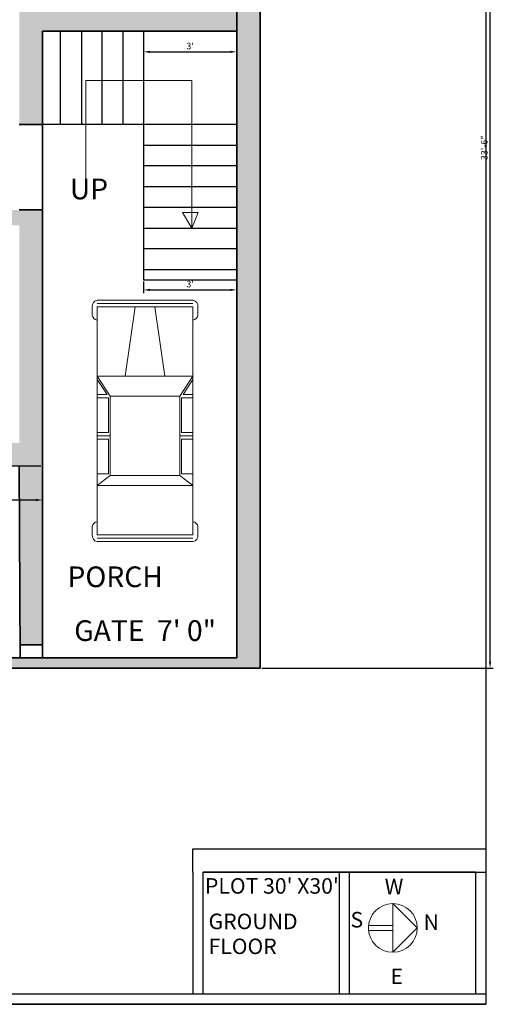
# Model space of a CAD drawing. Units: inches. Extents: x 2341 to 2872, y 1788 to 2419.
# Tile 2 of 3: x 2689 to 2872, y 1813 to 2194. Entities that reach past the tile are written whole.
import ezdxf

# ---------------------------------------------------------------- set-up
doc = ezdxf.new("R2010")
doc.units = ezdxf.units.IN
for name, color, linetype, lineweight in [('A-ANNO-DIMS', 2, 'Continuous', 18), ('A-ANNO-SYMB', 7, 'Continuous', 18), ('A-ANNO-TEXT', 7, 'Continuous', 25), ('A-ANNO-TTLB', 7, 'Continuous', 25), ('A-AREA-IDEN', 7, 'Continuous', 25), ('A-EQPM-VEHI', 8, 'Continuous', 13), ('A-FLOR-STRS', 7, 'Continuous', 25), ('A-WALL', 7, 'Continuous', 35)]:
    doc.layers.add(name, color=color, linetype=linetype, lineweight=lineweight)
doc.layers.add('A-WALL-PATT', color=18, linetype='Continuous', lineweight=13, true_color=0x000000)
doc.styles.get("Standard").update_dxf_attribs({"font": 'arial.ttf'})
doc.dimstyles.new('Copy of ISO-25', dxfattribs={"dimtxt": 2.5, "dimasz": 2.5, "dimexe": 1.25, "dimexo": 0.625, "dimtad": 1, "dimdec": 1, "dimlunit": 4, "dimtxsty": 'Standard', "dimcen": 2.5, "dimadec": 0, "dimazin": 0, "dimtfac": 1, "dimtdec": 1, "dimtmove": 0, "dimatfit": 3, "dimfxl": 1, "dimarcsym": 0})

# ---------------------------------------------------------------- blocks, each defined once
blk = doc.blocks.new('*U6')
for p, q in [((138, 1075), (308, 1075)), ((4818, 1075), (4649, 1075)), ((3, -10), (3, 974)), ((70, -10), (70, 973)), ((138, 973), (410, 973)), ((138, -10), (138, 971)), ((410, 973), (4581, 973)), ((1563, -10), (1563, 973)), ((1563, 973), (1969, 702)), ((1630, 973), (1936, 769)), ((1936, 769), (1936, 973)), ((2003, 973), (2003, 736)), ((2716, 736), (2716, 973)), ((2783, 702), (2783, 973)), ((2851, 973), (2851, 736)), ((3563, 736), (3563, 973)), ((3597, 702), (3801, 973)), ((3801, -10), (3801, 973)), ((4818, 973), (4547, 973)), ((4818, -10), (4818, 971)), ((4886, -10), (4886, 973)), ((4954, -10), (4954, 974)), ((1969, 702), (3597, 702)), ((1969, -10), (1969, 702)), ((2003, 736), (2716, 736)), ((2851, 736), (3563, 736)), ((3597, -10), (3597, 702)), ((138, 193), (1563, 396)), ((3, -11), (3, -995)), ((70, -10), (70, -994)), ((138, -11), (138, -992)), ((1563, -10), (1563, -994)), ((1969, -10), (1969, -723)), ((3597, -10), (3597, -723)), ((3801, -10), (3801, -994)), ((4818, -11), (4818, -992)), ((4886, -10), (4886, -994)), ((4954, -11), (4954, -995)), ((138, -214), (1563, -417)), ((1563, -994), (1969, -723)), ((1630, -994), (1936, -790)), ((1936, -790), (1936, -994)), ((1969, -723), (3597, -723)), ((2003, -994), (2003, -757)), ((2003, -757), (2716, -757)), ((2716, -757), (2716, -994)), ((2783, -723), (2783, -994)), ((2851, -757), (3563, -757)), ((2851, -994), (2851, -757)), ((3563, -757), (3563, -994)), ((3597, -723), (3801, -994)), ((138, -994), (410, -994)), ((410, -994), (4581, -994)), ((4818, -994), (4547, -994)), ((138, -1096), (308, -1096)), ((4818, -1096), (4649, -1096))]:
    blk.add_line(p, q)
for centre, radius, start, end in [((128, 946), 129, 85.6455, 168.0943), ((291, 956), 120, 8.1301, 81.87), ((4665, 956), 120, 98.13, 171.8699), ((4828, 946), 129, 11.9057, 94.3545), ((128, -967), 129, 191.9057, 274.3545), ((291, -977), 120, 278.13, 351.8699), ((4665, -977), 120, 188.1301, 261.87), ((4828, -967), 129, 265.6455, 348.0943)]:
    blk.add_arc(centre, radius, start, end)
blk = doc.blocks.new('*D21')
at = {"layer": 'A-ANNO-DIMS', "color": 0, "lineweight": -2, "transparency": 16777216}
for p, q in [((2556.55, 2020.39), (2556.55, 2006.73)), ((2697.55, 2020.39), (2697.55, 2006.73)), ((2559.05, 2007.98), (2695.05, 2007.98))]:
    blk.add_line(p, q, dxfattribs=at)
at = {"layer": 'A-ANNO-DIMS', "color": 0, "transparency": 16777216}
for points in [[(2559.05, 2008.4), (2559.05, 2007.57), (2556.55, 2007.98)], [(2695.05, 2008.4), (2695.05, 2007.57), (2697.55, 2007.98)]]:
    blk.add_solid(points, dxfattribs=at)
at = {"layer": 'Defpoints', "color": 0, "transparency": 16777216}
for p in [(2556.55, 2021.02), (2697.55, 2021.02), (2697.55, 2007.98)]:
    blk.add_point(p, dxfattribs=at)
at = {"layer": 'A-ANNO-DIMS', "color": 0, "transparency": 16777216, "insert": (2627.05, 2009.89), "char_height": 2.5, "attachment_point": 5}
blk.add_mtext('11\'-9"', dxfattribs=at)
blk = doc.blocks.new('*D22')
at = {"layer": 'A-ANNO-DIMS', "color": 0, "lineweight": -2, "transparency": 16777216}
for p, q in [((2696.93, 2021.02), (2680.85, 2021.02)), ((2682.1, 1949.52), (2682.1, 2018.52)), ((2696.93, 1947.02), (2680.85, 1947.02))]:
    blk.add_line(p, q, dxfattribs=at)
at = {"layer": 'A-ANNO-DIMS', "color": 0, "transparency": 16777216}
for points in [[(2681.68, 2018.52), (2682.52, 2018.52), (2682.1, 2021.02)], [(2681.68, 1949.52), (2682.52, 1949.52), (2682.1, 1947.02)]]:
    blk.add_solid(points, dxfattribs=at)
at = {"layer": 'Defpoints', "color": 0, "transparency": 16777216}
for p in [(2682.1, 2021.02), (2697.55, 2021.02), (2697.55, 1947.02)]:
    blk.add_point(p, dxfattribs=at)
at = {"layer": 'A-ANNO-DIMS', "color": 0, "transparency": 16777216, "insert": (2680.2, 1984.02), "char_height": 2.5, "attachment_point": 5, "rotation": 90}
blk.add_mtext('6\'-2"', dxfattribs=at)
blk = doc.blocks.new('*D27')
at = {"layer": 'A-ANNO-DIMS', "color": 0, "lineweight": -2, "transparency": 16777216}
for p, q in [((2736.55, 2092.39), (2736.55, 2087.89)), ((2772.55, 2092.39), (2772.55, 2087.89)), ((2739.05, 2089.14), (2770.05, 2089.14))]:
    blk.add_line(p, q, dxfattribs=at)
at = {"layer": 'A-ANNO-DIMS', "color": 0, "transparency": 16777216}
for points in [[(2739.05, 2089.56), (2739.05, 2088.72), (2736.55, 2089.14)], [(2770.05, 2089.56), (2770.05, 2088.72), (2772.55, 2089.14)]]:
    blk.add_solid(points, dxfattribs=at)
at = {"layer": 'Defpoints', "color": 0, "transparency": 16777216}
for p in [(2736.55, 2093.02), (2772.55, 2093.02), (2772.55, 2089.14)]:
    blk.add_point(p, dxfattribs=at)
at = {"layer": 'A-ANNO-DIMS', "color": 0, "transparency": 16777216, "insert": (2754.55, 2091.04), "char_height": 2.5, "attachment_point": 5}
blk.add_mtext("3'", dxfattribs=at)
blk = doc.blocks.new('*D28')
at = {"layer": 'A-ANNO-DIMS', "color": 0, "lineweight": -2, "transparency": 16777216}
for p, q in [((2736.55, 2188.39), (2736.55, 2179.85)), ((2772.55, 2188.39), (2772.55, 2179.85)), ((2739.05, 2181.1), (2770.05, 2181.1))]:
    blk.add_line(p, q, dxfattribs=at)
at = {"layer": 'A-ANNO-DIMS', "color": 0, "transparency": 16777216}
for points in [[(2739.05, 2181.51), (2739.05, 2180.68), (2736.55, 2181.1)], [(2770.05, 2181.51), (2770.05, 2180.68), (2772.55, 2181.1)]]:
    blk.add_solid(points, dxfattribs=at)
at = {"layer": 'Defpoints', "color": 0, "transparency": 16777216}
for p in [(2736.55, 2189.02), (2772.55, 2189.02), (2772.55, 2181.1)]:
    blk.add_point(p, dxfattribs=at)
at = {"layer": 'A-ANNO-DIMS', "color": 0, "transparency": 16777216, "insert": (2754.55, 2183), "char_height": 2.5, "attachment_point": 5}
blk.add_mtext("3'", dxfattribs=at)
blk = doc.blocks.new('*D35')
at = {"layer": 'A-ANNO-DIMS', "color": 0, "lineweight": -2, "transparency": 16777216}
for p, q in [((2782.18, 2345.02), (2871.62, 2345.02)), ((2870.37, 1945.52), (2870.37, 2342.52)), ((2782.18, 1943.02), (2871.62, 1943.02))]:
    blk.add_line(p, q, dxfattribs=at)
at = {"layer": 'A-ANNO-DIMS', "color": 0, "transparency": 16777216}
for points in [[(2869.95, 2342.52), (2870.78, 2342.52), (2870.37, 2345.02)], [(2869.95, 1945.52), (2870.78, 1945.52), (2870.37, 1943.02)]]:
    blk.add_solid(points, dxfattribs=at)
at = {"layer": 'Defpoints', "color": 0, "transparency": 16777216}
for p in [(2781.55, 2345.02), (2870.37, 2345.02), (2781.55, 1943.02)]:
    blk.add_point(p, dxfattribs=at)
at = {"layer": 'A-ANNO-DIMS', "color": 0, "transparency": 16777216, "insert": (2868.46, 2144.02), "char_height": 2.5, "attachment_point": 5, "rotation": 90}
blk.add_mtext('33\'-6"', dxfattribs=at)

msp = doc.modelspace()

# ---------------------------------------------------------------- hatches: boundary and pattern name
at = {"layer": 'A-WALL-PATT'}
h = msp.add_hatch(color=256, dxfattribs=at)
h.dxf.hatch_style = 1
h.paths.add_polyline_path([(2781.55, 2345.02), (2421.55, 2345.02), (2421.55, 1985.02), (2421.55, 1949.02), (2421.55, 1943.02), (2781.55, 1943.02), (2781.55, 1985.02)])
h.paths.add_polyline_path([(2550.55, 2336.02), (2772.55, 2336.02), (2772.55, 1994.02), (2772.55, 1985.02), (2772.55, 1947.02), (2430.55, 1947.02), (2430.55, 1985.02), (2454.55, 1985.02), (2454.55, 1994.02), (2430.55, 1994.02), (2430.55, 2114.02), (2496.55, 2114.02), (2514.55, 2114.02), (2514.55, 2120.02), (2496.55, 2120.02), (2496.55, 2168.02), (2556.55, 2168.02), (2556.55, 2174.02), (2550.55, 2174.02), (2478.55, 2174.02), (2478.55, 2170.02), (2490.55, 2170.02), (2490.55, 2168.02), (2490.55, 2120.02), (2430.55, 2120.02), (2430.55, 2168.02), (2430.55, 2174.02), (2430.55, 2204.02), (2430.55, 2336.02)], flags=16)
h.paths.add_polyline_path([(2556.55, 2336.02), (2652.55, 2336.02), (2652.55, 2198.02), (2646.55, 2198.02), (2601.55, 2198.02), (2595.55, 2198.02), (2595.55, 2240.02), (2556.55, 2240.02), (2556.55, 2246.02), (2556.55, 2294.02)], flags=0)
h.paths.add_polyline_path([(2556.55, 2300.02), (2646.55, 2300.02), (2646.55, 2294.02), (2646.55, 2204.02), (2601.55, 2204.02), (2601.55, 2246.02), (2601.55, 2294.02), (2613.55, 2294.02), (2613.55, 2300.02), (2592.55, 2300.02), (2592.55, 2294.02), (2595.55, 2294.02), (2595.55, 2246.02), (2556.55, 2246.02), (2556.55, 2282.02)], flags=0)
h.paths.add_polyline_path([(2680.26, 2307.06), (2747.77, 2307.06), (2747.77, 2329.57), (2770.28, 2329.57), (2770.28, 2307.06), (2770.28, 2239.54), (2770.28, 2217.04), (2747.77, 2217.04), (2747.77, 2239.54), (2680.26, 2239.54)], flags=0)
h.paths.add_polyline_path([(2681.16, 2306.16), (2769.38, 2306.16), (2769.38, 2240.44), (2704.56, 2240.44, -0.009128), (2703.54, 2240.44), (2681.16, 2240.44)], flags=0)
h.paths.add_polyline_path([(2744.14, 2298.19), (2744.14, 2293.47), (2696.44, 2293.47), (2696.44, 2242.73, -0.092104), (2691.71, 2247), (2691.71, 2298.19)], flags=0)
h.paths.add_polyline_path([(2694.86, 2296.62), (2694.86, 2295.04), (2693.29, 2295.04), (2693.29, 2296.62)], flags=0)
h.paths.add_polyline_path([(2478.55, 2173.02), (2478.55, 2172.02), (2478.55, 2171.02), (2442.55, 2171.02), (2442.55, 2170.02), (2438.98, 2170.02), (2430.55, 2170.02), (2430.55, 2174.02), (2442.55, 2174.02), (2442.55, 2173.02)], flags=0)
h.paths.add_polyline_path([(2688.55, 2198.02), (2697.55, 2198.02), (2772.55, 2198.02), (2772.55, 2189.02), (2772.55, 2153.02), (2755.26, 2153.02), (2755.26, 2145.02), (2772.55, 2145.02), (2772.55, 2137.02), (2755.26, 2137.02), (2755.26, 2129.02), (2772.55, 2129.02), (2772.55, 2121.02), (2755.26, 2121.02), (2755.26, 2119.07), (2757.66, 2119.07), (2755.26, 2113.02), (2772.55, 2113.02), (2772.55, 2105.02), (2736.55, 2105.02), (2736.55, 2153.02), (2697.55, 2153.02), (2697.55, 2021.02), (2697.55, 1952.02), (2688.89, 1952.02), (2688.89, 1947.02), (2688.59, 2021.02), (2688.55, 2021.02), (2580.55, 2021.02), (2580.55, 2030.02), (2556.55, 2030.02), (2556.55, 2114.02), (2580.55, 2114.02), (2580.55, 2120.02), (2664.55, 2120.02), (2688.55, 2120.02), (2688.55, 2189.02)], flags=0)
h.paths.add_polyline_path([(2510.86, 2109.17, -0.414214), (2512.75, 2107.25), (2512.59, 2085.13, -0.414214), (2511.43, 2083.99), (2508, 2084.02, -0.414214), (2506.86, 2085.17), (2487.78, 2085.31, -0.414214), (2485.88, 2087.24, -0.414214), (2483.96, 2085.34), (2464.87, 2085.49, -0.414214), (2462.98, 2087.41, -0.414214), (2461.06, 2085.52), (2441.97, 2085.66, -0.414214), (2440.82, 2084.52), (2437.38, 2084.55, -0.414214), (2436.25, 2085.7), (2436.41, 2107.83, -0.414214), (2438.34, 2109.72)], flags=0)
h.paths.add_polyline_path([(2736.55, 2189.02), (2736.55, 2170), (2728.55, 2170), (2728.55, 2153.02), (2720.55, 2153.02), (2720.55, 2189.02), (2712.55, 2189.02), (2712.55, 2153.02), (2704.55, 2153.02), (2704.55, 2189.02)], flags=0)
edge = h.paths.add_edge_path(flags=0)
edge.add_ellipse((2759.52, 2317.47), major_axis=(6.08, 0), ratio=0.975448, start_angle=450, end_angle=540, ccw=False)
edge.add_ellipse((2759.52, 2317.47), major_axis=(6.08, 0), ratio=0.975448, start_angle=360, end_angle=450, ccw=False)
edge.add_ellipse((2759.52, 2317.47), major_axis=(6.08, 0), ratio=0.975448, start_angle=270, end_angle=360, ccw=False)
edge.add_ellipse((2759.52, 2317.47), major_axis=(6.08, 0), ratio=0.975448, start_angle=180, end_angle=270, ccw=False)
h.paths.add_polyline_path([(2505.86, 2104.26, -0.414214), (2507, 2103.11), (2506.89, 2089.02), (2442, 2089.51), (2442.11, 2103.6, -0.414214), (2443.26, 2104.74)], flags=0)
h.paths.add_polyline_path([(2485.9, 2089.94), (2463, 2090.11), (2463.01, 2091.64), (2485.91, 2091.47)], flags=0)
h.paths.add_polyline_path([(2758.23, 2298.35), (2764.61, 2298.35, -0.414214), (2768.21, 2294.75), (2768.21, 2280.47, -0.414214), (2764.61, 2276.87), (2758.23, 2276.87, -0.414214), (2754.62, 2280.47), (2754.62, 2294.75, -0.414214)], flags=0)
h.paths.add_polyline_path([(2758.23, 2297.45), (2764.61, 2297.45, -0.414214), (2767.31, 2294.75), (2767.31, 2280.47, -0.414214), (2764.61, 2277.77), (2758.23, 2277.77, -0.414214), (2755.52, 2280.47), (2755.52, 2294.75, -0.414214)], flags=0)
h.paths.add_polyline_path([(2758.23, 2265.42), (2764.61, 2265.42, -0.414214), (2768.21, 2261.82), (2768.21, 2247.53, -0.414214), (2764.61, 2243.93), (2758.23, 2243.93, -0.414214), (2754.62, 2247.53), (2754.62, 2261.82, -0.414214)], flags=0)
h.paths.add_polyline_path([(2758.23, 2264.52), (2764.61, 2264.52, -0.414214), (2767.31, 2261.82), (2767.31, 2247.53, -0.414214), (2764.61, 2244.83), (2758.23, 2244.83, -0.414214), (2755.52, 2247.53), (2755.52, 2261.82, -0.414214)], flags=0)
edge = h.paths.add_edge_path(flags=0)
edge.add_ellipse((2759.52, 2229.13), major_axis=(6.08, 0), ratio=0.975448, start_angle=90, end_angle=180, ccw=False)
edge.add_ellipse((2759.52, 2229.13), major_axis=(6.08, 0), ratio=0.975448, start_angle=0, end_angle=90, ccw=False)
edge.add_ellipse((2759.52, 2229.13), major_axis=(6.08, 0), ratio=0.975448, start_angle=270, end_angle=360, ccw=False)
edge.add_ellipse((2759.52, 2229.13), major_axis=(6.08, 0), ratio=0.975448, start_angle=180, end_angle=270, ccw=False)
h.paths.add_polyline_path([(2457.94, 2073.59, -0.414214), (2459.08, 2072.44), (2459.05, 2069, -0.414214), (2457.9, 2067.87), (2457.75, 2048.78, -0.414214), (2455.83, 2046.89, -0.414214), (2457.72, 2044.96), (2457.58, 2025.88, -0.414214), (2455.66, 2023.98, -0.414214), (2457.55, 2022.06), (2457.41, 2002.98, -0.414214), (2458.54, 2001.82), (2458.52, 1998.39, -0.414214), (2457.36, 1997.25), (2435.24, 1997.42, -0.414214), (2433.35, 1999.34), (2433.89, 2071.86, -0.414214), (2435.82, 2073.76)], flags=0)
h.paths.add_polyline_path([(2454.05, 2067.89), (2453.56, 2003), (2439.47, 2003.11, -0.414214), (2438.33, 2004.26), (2438.8, 2066.86, -0.414214), (2439.96, 2068)], flags=0)
h.paths.add_polyline_path([(2452.95, 2024), (2451.43, 2024.02), (2451.6, 2046.92), (2453.13, 2046.91)], flags=0)
h.paths.add_polyline_path([(2830.4, 1819.46), (2838.99, 1819.46), (2838.99, 1828.46), (2830.4, 1828.46)], flags=9)
h.paths.add_polyline_path([(2814.93, 1841.19), (2823.62, 1841.19), (2823.62, 1850.5), (2814.93, 1850.5)], flags=9)
h.paths.add_polyline_path([(2843.19, 1840.36), (2852.25, 1840.36), (2852.25, 1849.36), (2843.19, 1849.36)], flags=9)
h.paths.add_polyline_path([(2828.19, 1854.15), (2839.1, 1854.15), (2839.1, 1863.15), (2828.19, 1863.15)], flags=9)
h.paths.add_polyline_path([(2760.12, 1830.89), (2792.1, 1830.89), (2792.1, 1840.21), (2760.12, 1840.21)], flags=9)
h.paths.add_polyline_path([(2760.12, 1840.53), (2800.48, 1840.53), (2800.48, 1849.85), (2760.12, 1849.85)], flags=9)
h.paths.add_polyline_path([(2758.73, 1854.24), (2815.82, 1854.24), (2815.82, 1863.56), (2758.73, 1863.56)], flags=9)
h.paths.add_polyline_path([(2482.08, 1917.73), (2536.72, 1917.73), (2536.72, 1936.36), (2482.08, 1936.36)], flags=9)
h.paths.add_polyline_path([(2707.72, 1951.32), (2770.13, 1951.32), (2770.13, 1963.73), (2707.72, 1963.73)], flags=8)
h.paths.add_polyline_path([(2706.05, 2121.97), (2725.65, 2121.97), (2725.65, 2134.17), (2706.05, 2134.17)], flags=8)
h.paths.add_polyline_path([(2705.12, 1972.11), (2749.62, 1972.11), (2749.62, 1984.52), (2705.12, 1984.52)], flags=8)
h.paths.add_polyline_path([(2468.66, 1961.36), (2524.36, 1961.36), (2524.36, 1973.77), (2468.66, 1973.77)], flags=8)
h.paths.add_polyline_path([(2572.95, 1988.2), (2639.05, 1988.2), (2639.05, 2000.2), (2572.95, 2000.2)], flags=8)
h.paths.add_polyline_path([(2460.85, 2050.66), (2556.87, 2050.66), (2556.87, 2063.08), (2460.85, 2063.08)], flags=8)
h.paths.add_polyline_path([(2575.44, 2073.64), (2628.63, 2073.64), (2628.63, 2086.04), (2575.44, 2086.04)], flags=8)
h.paths.add_polyline_path([(2575.12, 2153.95), (2616.53, 2153.95), (2616.53, 2166.37), (2575.12, 2166.37)], flags=8)
h.paths.add_polyline_path([(2664.33, 2218.95), (2729.32, 2218.95), (2729.32, 2231.37), (2664.33, 2231.37)], flags=8)
h.paths.add_polyline_path([(2557.77, 2265.61), (2586.74, 2265.61), (2586.74, 2278.02), (2557.77, 2278.02)], flags=8)
h.paths.add_polyline_path([(2605.48, 2263.57), (2639.29, 2263.57), (2639.29, 2275.57), (2605.48, 2275.57)], flags=8)
h.paths.add_polyline_path([(2569.54, 2309.66), (2602.87, 2309.66), (2602.87, 2322.07), (2569.54, 2322.07)], flags=8)
h.paths.add_polyline_path([(2458.16, 2214.67), (2523.15, 2214.67), (2523.15, 2227.09), (2458.16, 2227.09)], flags=8)
h.paths.add_polyline_path([(2458.16, 2227.52), (2511.98, 2227.52), (2511.98, 2239.93), (2458.16, 2239.93)], flags=8)
h.paths.add_polyline_path([(2449.57, 2140.97), (2449.57, 2149.18), (2444.42, 2149.18), (2444.42, 2140.97)], flags=8)
h.paths.add_polyline_path([(2458.63, 2128.07), (2462.49, 2128.07), (2462.49, 2133.23), (2458.63, 2133.23)], flags=8)
h.paths.add_polyline_path([(2506.29, 2142.15), (2506.29, 2146.01), (2501.14, 2146.01), (2501.14, 2142.15)], flags=8)
h.paths.add_polyline_path([(2487.54, 2002.8), (2493.34, 2002.8), (2493.34, 2007.95), (2487.54, 2007.95)], flags=8)
h.paths.add_polyline_path([(2479.27, 2051.01), (2479.27, 2056.81), (2474.12, 2056.81), (2474.12, 2051.01)], flags=8)
h.paths.add_polyline_path([(2441.47, 1961.92), (2441.47, 1970.13), (2436.31, 1970.13), (2436.31, 1961.92)], flags=8)
h.paths.add_polyline_path([(2682.8, 1979.93), (2682.8, 1988.13), (2677.65, 1988.13), (2677.65, 1979.93)], flags=8)
h.paths.add_polyline_path([(2752.63, 2088.44), (2756.49, 2088.44), (2756.49, 2093.6), (2752.63, 2093.6)], flags=8)
h.paths.add_polyline_path([(2752.63, 2180.4), (2756.49, 2180.4), (2756.49, 2185.55), (2752.63, 2185.55)], flags=8)
h.paths.add_polyline_path([(2740.86, 2261.83), (2740.86, 2271.98), (2735.71, 2271.98), (2735.71, 2261.83)], flags=8)
h.paths.add_polyline_path([(2709.54, 2328.87), (2715.34, 2328.87), (2715.34, 2334.02), (2709.54, 2334.02)], flags=8)
h.paths.add_polyline_path([(2639.95, 2316.1), (2639.95, 2319.95), (2634.8, 2319.95), (2634.8, 2316.1)], flags=8)
h.paths.add_polyline_path([(2597.45, 2328.64), (2605.65, 2328.64), (2605.65, 2333.8), (2597.45, 2333.8)], flags=8)
h.paths.add_polyline_path([(2487.54, 2325.01), (2493.34, 2325.01), (2493.34, 2330.16), (2487.54, 2330.16)], flags=8)
h.paths.add_polyline_path([(2541.67, 2249.83), (2541.67, 2259.98), (2536.52, 2259.98), (2536.52, 2249.83)], flags=8)
h = msp.add_hatch(color=256, dxfattribs=at)
h.dxf.hatch_style = 1
h.paths.add_polyline_path([(2556.55, 1994.02), (2556.55, 2021.02), (2580.55, 2021.02), (2580.55, 2030.02), (2556.55, 2030.02), (2556.55, 2114.02), (2580.55, 2114.02), (2580.55, 2120.02), (2556.55, 2120.02), (2550.55, 2120.02), (2550.55, 2114.02), (2550.55, 1994.02), (2526.55, 1994.02), (2526.55, 1985.02), (2556.55, 1985.02)])
h.paths.add_polyline_path([(2697.55, 2120.02), (2688.55, 2120.02), (2664.55, 2120.02), (2664.55, 2114.02), (2688.55, 2114.02), (2688.55, 2030.02), (2664.55, 2030.02), (2664.55, 2021.02), (2688.55, 2021.02), (2688.59, 2021.02), (2688.87, 1952.02), (2697.55, 1952.02), (2697.55, 2021.02)])
h.paths.add_polyline_path([(2772.55, 2198.02), (2688.55, 2198.02), (2688.55, 2189.02), (2688.55, 2153.02), (2697.55, 2153.02), (2697.55, 2189.02), (2772.55, 2189.02)])
h.paths.add_polyline_path([(2652.55, 2336.02), (2646.55, 2336.02), (2646.55, 2204.02), (2601.55, 2204.02), (2601.55, 2246.02), (2601.55, 2294.02), (2613.55, 2294.02), (2613.55, 2296.02), (2634.55, 2296.02), (2634.55, 2294.02), (2646.55, 2294.02), (2646.55, 2300.02), (2646.55, 2336.02), (2556.55, 2336.02), (2556.55, 2294.02), (2568.55, 2294.02), (2568.55, 2296.02), (2592.55, 2296.02), (2592.55, 2294.02), (2595.55, 2294.02), (2595.55, 2246.02), (2556.55, 2246.02), (2556.55, 2240.02), (2595.55, 2240.02), (2595.55, 2198.02), (2601.55, 2198.02), (2646.55, 2198.02), (2652.55, 2198.02)])
h.paths.add_polyline_path([(2442.55, 2174.02), (2430.55, 2174.02), (2430.55, 2170.02), (2442.55, 2170.02)])
h.paths.add_polyline_path([(2478.55, 2172.02), (2478.55, 2173.02), (2442.55, 2173.02), (2442.55, 2171.02), (2478.55, 2171.02)])
h.paths.add_polyline_path([(2556.55, 2336.02), (2550.55, 2336.02), (2550.55, 2210.02), (2556.55, 2210.02)])
h.paths.add_polyline_path([(2460.85, 2050.66), (2556.87, 2050.66), (2556.87, 2063.08), (2460.85, 2063.08)], flags=9)
h.paths.add_polyline_path([(2569.54, 2309.66), (2602.87, 2309.66), (2602.87, 2322.07), (2569.54, 2322.07)], flags=24)

# ---------------------------------------------------------------- linework, layer by layer
at = {"layer": 'A-ANNO-SYMB'}
for p, q in [((2714.32, 2132), (2714.32, 2170)), ((2714.32, 2170), (2755.26, 2170)), ((2755.26, 2170), (2755.26, 2113.02)), ((2755.26, 2113.02), (2751.57, 2119.07)), ((2751.57, 2119.07), (2757.66, 2119.07)), ((2755.26, 2113.02), (2757.66, 2119.07)), ((2832.82, 1843.67), (2832.82, 1852.07)), ((2832.82, 1852.07), (2842.22, 1842.67)), ((2823.46, 1843.6), (2823.42, 1842.67)), ((2823.42, 1842.67), (2823.42, 1841.67)), ((2823.42, 1841.67), (2832.82, 1841.67)), ((2832.82, 1843.67), (2823.46, 1843.6)), ((2832.82, 1842.67), (2832.82, 1843.67)), ((2832.82, 1841.67), (2832.82, 1842.67)), ((2832.82, 1842.67), (2832.82, 1833.27)), ((2832.82, 1833.27), (2842.22, 1842.67))]:
    msp.add_line(p, q, dxfattribs=at)
msp.add_circle((2832.82, 1842.67), 9.4, dxfattribs=at)
at = {"layer": 'A-ANNO-TTLB'}
for p, q in [((2755.61, 1873.17), (2868.69, 1873.17)), ((2755.61, 1864.17), (2755.61, 1873.17)), ((2755.61, 1864.17), (2755.61, 1817.17)), ((2864.69, 1864.17), (2759.61, 1864.17)), ((2759.61, 1817.17), (2759.61, 1864.17)), ((2759.61, 1864.17), (2868.69, 1864.17)), ((2812.15, 1864.17), (2812.15, 1817.17)), ((2816.15, 1817.17), (2816.15, 1864.17)), ((2864.69, 1864.17), (2864.69, 1817.17)), ((2868.69, 1864.17), (2868.69, 1817.17)), ((2341.19, 1817.17), (2868.69, 1817.17)), ((2755.61, 1817.17), (2759.61, 1817.17)), ((2812.15, 1817.17), (2816.15, 1817.17)), ((2341.19, 1813.17), (2868.69, 1813.17))]:
    msp.add_line(p, q, dxfattribs=at)
msp.add_lwpolyline([(2341.19, 2419.31), (2868.69, 2419.31), (2868.69, 1813.17), (2341.19, 1813.17)], close=True, dxfattribs=at)
at = {"layer": 'A-FLOR-STRS'}
for p, q in [((2704.55, 2153.02), (2704.55, 2189.02)), ((2720.55, 2189.02), (2712.55, 2189.02)), ((2712.55, 2189.02), (2712.55, 2153.02)), ((2720.55, 2153.02), (2720.55, 2189.02)), ((2736.55, 2189.02), (2728.55, 2189.02)), ((2728.55, 2189.02), (2728.55, 2153.02)), ((2772.55, 2189.02), (2736.55, 2189.02)), ((2736.55, 2189.02), (2736.55, 2153.02)), ((2772.55, 2189.02), (2772.55, 2153.02)), ((2772.55, 2153.02), (2697.55, 2153.02)), ((2712.55, 2153.02), (2704.55, 2153.02)), ((2728.55, 2153.02), (2720.55, 2153.02)), ((2736.55, 2153.02), (2736.55, 2093.02)), ((2736.55, 2153.02), (2736.55, 2145.02)), ((2736.55, 2145.02), (2772.55, 2145.02)), ((2772.55, 2145.02), (2772.55, 2137.02)), ((2772.55, 2137.02), (2736.55, 2137.02)), ((2736.55, 2137.02), (2736.55, 2129.02)), ((2736.55, 2129.02), (2772.55, 2129.02)), ((2772.55, 2129.02), (2772.55, 2121.02)), ((2772.55, 2121.02), (2736.55, 2121.02)), ((2736.55, 2121.02), (2736.55, 2113.02)), ((2736.55, 2113.02), (2772.55, 2113.02)), ((2772.55, 2113.02), (2772.55, 2105.02)), ((2772.55, 2105.02), (2736.55, 2105.02)), ((2736.55, 2105.02), (2736.55, 2097.02)), ((2736.55, 2097.02), (2772.55, 2097.02)), ((2772.55, 2097.02), (2772.55, 2097.02)), ((2736.55, 2093.02), (2772.55, 2093.02))]:
    msp.add_line(p, q, dxfattribs=at)
at = {"layer": 'A-WALL'}
for p, q in [((2781.55, 2345.02), (2781.55, 1985.02)), ((2772.55, 2198.02), (2772.55, 2189.02)), ((2772.55, 2189.02), (2697.55, 2189.02)), ((2697.55, 2189.02), (2697.55, 2021.02)), ((2697.55, 2153.02), (2688.55, 2153.02)), ((2688.55, 2120.02), (2697.55, 2120.02)), ((2688.59, 2021.02), (2688.89, 1947.02)), ((2697.55, 2021.02), (2697.55, 1947.02)), ((2772.55, 1994.02), (2772.55, 1985.02)), ((2772.55, 1985.02), (2772.55, 1947.02)), ((2781.55, 1943.02), (2781.55, 1985.02)), ((2688.89, 1947.02), (2688.89, 1952.02)), ((2688.89, 1952.02), (2697.55, 1952.02)), ((2430.55, 1947.02), (2772.55, 1947.02)), ((2421.55, 1943.02), (2781.55, 1943.02))]:
    msp.add_line(p, q, dxfattribs=at)
for points in [[(2421.55, 1985.02), (2421.55, 2345.02), (2781.55, 2345.02), (2781.55, 1985.02)], [(2430.55, 2174.02), (2430.55, 2336.02), (2772.55, 2336.02), (2772.55, 1994.02)]]:
    msp.add_lwpolyline(points, dxfattribs=at)

# ---------------------------------------------------------------- block references
at = {"layer": 'A-EQPM-VEHI', "xscale": 0.018830901400966, "yscale": 0.018830901400966, "zscale": 0.018830901400966, "rotation": 270}
msp.add_blockref('*U6', (2737.33, 2085.2), dxfattribs=at)

# ---------------------------------------------------------------- texts
at = {"layer": 'A-ANNO-SYMB'}
for s, p in [('W', (2829.69, 1855.65)), ('S', (2816.48, 1842.85)), ('N', (2844.69, 1841.86)), ('E', (2831.9, 1820.96))]:
    msp.add_text(s, height=6, dxfattribs=at).set_placement(p)
at = {"layer": 'A-ANNO-TEXT'}
for s, p in [('UP', (2708.09, 2124.14)), ('GATE  7\' 0"', (2709.78, 1953.52))]:
    msp.add_text(s, height=8, dxfattribs=at).set_placement(p)
at = {"layer": 'A-ANNO-TTLB'}
for s, p in [("PLOT 30' X30'", (2760.28, 1855.9)), ('GROUND', (2761.67, 1842.19)), ('FLOOR', (2761.67, 1832.55))]:
    msp.add_text(s, height=6, dxfattribs=at).set_placement(p)
at = {"layer": 'A-AREA-IDEN'}
msp.add_text('PORCH', height=8, dxfattribs=at).set_placement((2707.19, 1974.31))

# ---------------------------------------------------------------- dimensions: what is measured, and where the dimension line sits
at = {"layer": 'A-ANNO-DIMS'}
for base, p1, p2, override, picture, middle in [((2870.37, 2345.02), (2781.55, 1943.02), (2781.55, 2345.02), {"dimdec": 1, "dimlfac": 1, "dimrnd": 0, "dimzin": 1, "dimdsep": 46, "dimlunit": 4, "dimfrac": 2}, '*D35', (2868.46, 2144.02)), ((2682.1, 2021.02), (2697.55, 1947.02), (2697.55, 2021.02), {"dimclrd": 0, "dimclre": 0, "dimclrt": 0}, '*D22', (2680.2, 1984.02))]:
    dim = msp.add_linear_dim(base=base, p1=p1, p2=p2, angle=90, dimstyle='Copy of ISO-25', override=override, dxfattribs=at)
    dim.commit()
    dim.dimension.update_dxf_attribs({"geometry": picture, "text_midpoint": middle})
for base, p1, p2, picture, middle in [((2772.55, 2181.1), (2736.55, 2189.02), (2772.55, 2189.02), '*D28', (2754.55, 2183)), ((2772.55, 2089.14), (2736.55, 2093.02), (2772.55, 2093.02), '*D27', (2754.55, 2091.04)), ((2697.55, 2007.98), (2556.55, 2021.02), (2697.55, 2021.02), '*D21', (2627.05, 2009.89))]:
    dim = msp.add_linear_dim(base=base, p1=p1, p2=p2, dimstyle='Copy of ISO-25', override={"dimclrd": 0, "dimclre": 0, "dimclrt": 0}, dxfattribs=at)
    dim.commit()
    dim.dimension.update_dxf_attribs({"geometry": picture, "text_midpoint": middle})

doc.saveas('drawing.dxf')
